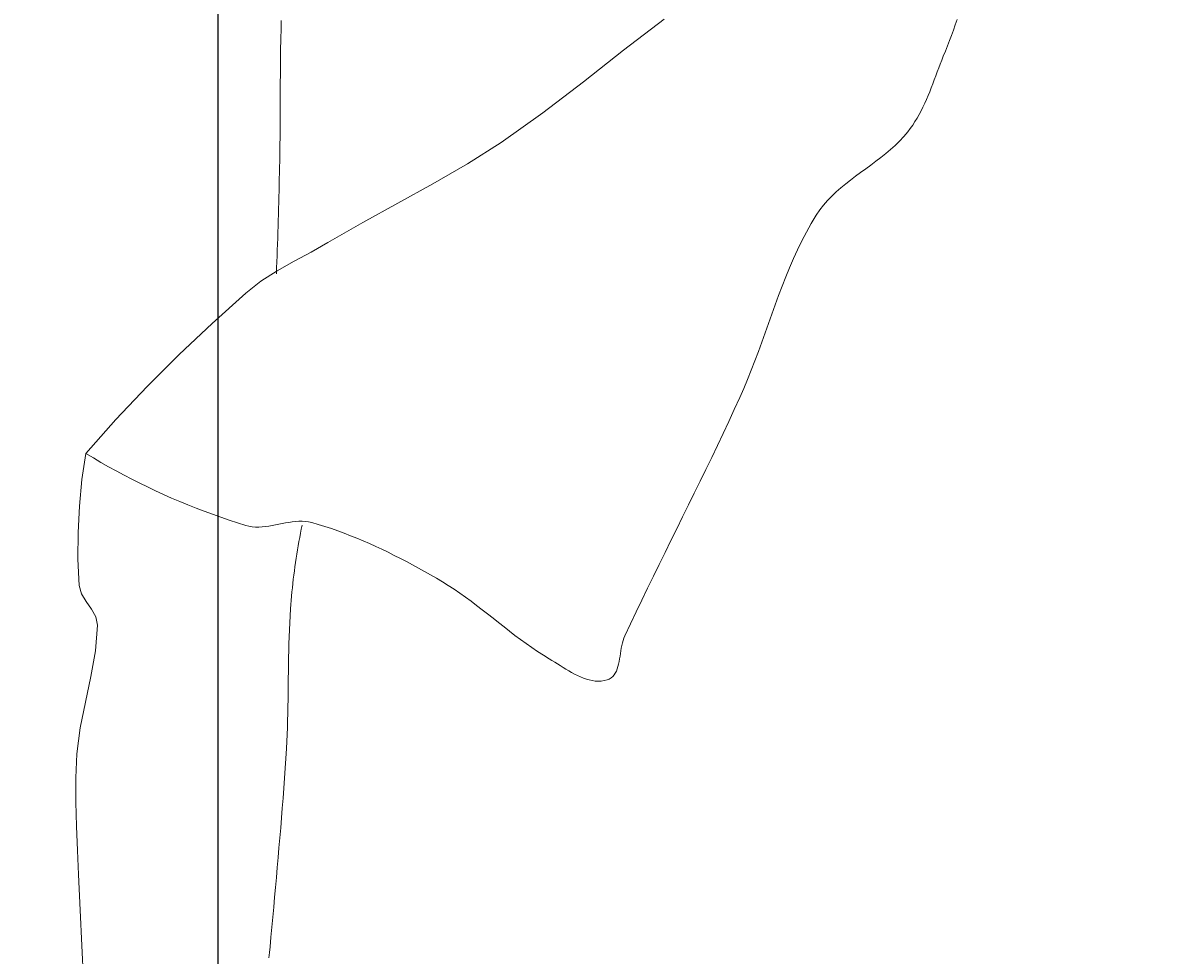
# Model space of a CAD drawing. Units: inches. Extents: x 1770 to 2988, y 1161 to 3221.
# Tile 25 of 44: x 2524 to 2562, y 2300 to 2330. Entities that reach past the tile are written whole.
import ezdxf

# ---------------------------------------------------------------- set-up
doc = ezdxf.new("R2010")
doc.units = ezdxf.units.IN
doc.layers.add('A-ANNO-DIMS', color=2, linetype='Continuous', lineweight=18)
doc.layers.add('A-FURN', color=8, linetype='Continuous', lineweight=13)
doc.styles.get("Standard").update_dxf_attribs({"font": 'arial.ttf'})
doc.dimstyles.get("Standard").update_dxf_attribs({"dimtxt": 0.18, "dimasz": 0.18, "dimexe": 0.18, "dimexo": 0.0625, "dimgap": 0.09, "dimtad": 0, "dimtih": 1, "dimtoh": 1, "dimdec": 4, "dimzin": 0, "dimdsep": 46, "dimtxsty": 'Standard', "dimcen": 0.09, "dimadec": 0, "dimazin": 0, "dimtfac": 1, "dimtdec": 4, "dimtofl": 0, "dimtmove": 0, "dimatfit": 3, "dimfxl": 1, "dimtolj": 1, "dimtzin": 0, "dimarcsym": 0})

# ---------------------------------------------------------------- blocks, each defined once
blk = doc.blocks.new('BED-DOUBLE-PLAN')
for p, q in [((6.794, 74.245), (6.798, 74.421)), ((6.798, 74.421), (6.803, 74.596)), ((19.481, 74.65), (18.14, 73.617)), ((29.058, 74.282), (29.122, 74.456)), ((29.122, 74.456), (29.185, 74.63)), ((6.786, 73.894), (6.79, 74.07)), ((6.79, 74.07), (6.794, 74.245)), ((28.927, 73.935), (28.993, 74.108)), ((28.993, 74.108), (29.058, 74.282)), ((6.779, 73.519), (6.782, 73.706)), ((6.782, 73.706), (6.786, 73.894)), ((28.792, 73.59), (28.86, 73.762)), ((28.86, 73.762), (28.927, 73.935)), ((6.775, 73.143), (6.777, 73.331)), ((6.777, 73.331), (6.779, 73.519)), ((18.14, 73.617), (16.81, 72.571)), ((28.623, 73.159), (28.673, 73.289)), ((28.673, 73.289), (28.724, 73.417)), ((28.724, 73.417), (28.792, 73.59)), ((6.772, 72.768), (6.773, 72.955)), ((6.773, 72.955), (6.775, 73.143)), ((28.476, 72.767), (28.525, 72.898)), ((28.525, 72.898), (28.574, 73.028)), ((28.574, 73.028), (28.623, 73.159)), ((6.77, 72.392), (6.771, 72.58)), ((6.771, 72.58), (6.772, 72.768)), ((16.81, 72.571), (15.466, 71.543)), ((28.327, 72.374), (28.377, 72.504)), ((28.377, 72.504), (28.427, 72.635)), ((28.427, 72.635), (28.476, 72.767)), ((6.769, 72.204), (6.77, 72.392)), ((6.769, 72.017), (6.769, 72.204)), ((28.168, 71.987), (28.222, 72.115)), ((28.222, 72.115), (28.275, 72.244)), ((28.275, 72.244), (28.327, 72.374)), ((6.767, 71.641), (6.768, 71.829)), ((6.768, 71.829), (6.769, 72.017)), ((27.99, 71.61), (28.052, 71.734)), ((28.052, 71.734), (28.111, 71.86)), ((28.111, 71.86), (28.168, 71.987)), ((6.766, 71.266), (6.767, 71.453)), ((6.767, 71.453), (6.767, 71.641)), ((15.466, 71.543), (14.086, 70.565)), ((27.786, 71.251), (27.858, 71.368)), ((27.858, 71.368), (27.926, 71.488)), ((27.926, 71.488), (27.99, 71.61)), ((6.763, 70.89), (6.765, 71.078)), ((6.765, 71.078), (6.766, 71.266)), ((27.547, 70.914), (27.631, 71.023)), ((27.631, 71.023), (27.711, 71.136)), ((27.711, 71.136), (27.786, 71.251)), ((6.759, 70.515), (6.762, 70.702)), ((6.762, 70.702), (6.763, 70.89)), ((27.128, 70.466), (27.275, 70.609)), ((27.275, 70.609), (27.415, 70.757)), ((27.415, 70.757), (27.547, 70.914)), ((6.754, 70.139), (6.757, 70.327)), ((6.757, 70.327), (6.759, 70.515)), ((14.086, 70.565), (12.968, 69.855)), ((26.817, 70.196), (26.975, 70.328)), ((26.975, 70.328), (27.128, 70.466)), ((6.746, 69.747), (6.75, 69.943)), ((6.75, 69.943), (6.754, 70.139)), ((12.968, 69.855), (11.823, 69.189)), ((26.324, 69.815), (26.491, 69.94)), ((26.491, 69.94), (26.655, 70.066)), ((26.655, 70.066), (26.817, 70.196)), ((6.737, 69.355), (6.742, 69.551)), ((6.742, 69.551), (6.746, 69.747)), ((25.82, 69.445), (25.988, 69.569)), ((25.988, 69.569), (26.156, 69.692)), ((26.156, 69.692), (26.324, 69.815)), ((6.728, 68.962), (6.733, 69.158)), ((6.733, 69.158), (6.737, 69.355)), ((11.823, 69.189), (10.663, 68.547)), ((25.335, 69.061), (25.493, 69.192)), ((25.493, 69.192), (25.655, 69.319)), ((25.655, 69.319), (25.82, 69.445)), ((6.718, 68.57), (6.723, 68.766)), ((6.723, 68.766), (6.728, 68.962)), ((24.892, 68.64), (25.033, 68.785)), ((25.033, 68.785), (25.181, 68.926)), ((25.181, 68.926), (25.335, 69.061)), ((6.708, 68.178), (6.713, 68.374)), ((6.713, 68.374), (6.718, 68.57)), ((10.663, 68.547), (9.501, 67.907)), ((24.52, 68.158), (24.635, 68.327)), ((24.635, 68.327), (24.759, 68.487)), ((24.759, 68.487), (24.892, 68.64)), ((6.696, 67.786), (6.702, 67.982)), ((6.702, 67.982), (6.708, 68.178)), ((24.35, 67.879), (24.52, 68.158)), ((6.684, 67.394), (6.69, 67.59)), ((6.69, 67.59), (6.696, 67.786)), ((9.501, 67.907), (8.35, 67.249)), ((24.039, 67.305), (24.19, 67.594)), ((24.19, 67.594), (24.35, 67.879)), ((6.671, 67.001), (6.678, 67.198)), ((6.678, 67.198), (6.684, 67.394)), ((8.35, 67.249), (7.792, 66.934)), ((23.895, 67.012), (24.039, 67.305)), ((6.657, 66.609), (6.664, 66.805)), ((6.664, 66.805), (6.671, 67.001)), ((7.792, 66.934), (7.227, 66.627)), ((23.759, 66.715), (23.895, 67.012)), ((6.65, 66.413), (6.657, 66.609)), ((7.227, 66.627), (6.669, 66.31)), ((23.629, 66.414), (23.759, 66.715)), ((6.669, 66.31), (6.131, 65.965)), ((6.643, 66.217), (6.65, 66.413)), ((23.385, 65.806), (23.505, 66.111)), ((23.505, 66.111), (23.629, 66.414)), ((6.131, 65.965), (5.627, 65.574)), ((23.268, 65.499), (23.385, 65.806)), ((5.627, 65.574), (4.51, 64.573)), ((23.155, 65.19), (23.268, 65.499)), ((23.043, 64.88), (23.155, 65.19)), ((4.51, 64.573), (3.42, 63.541)), ((22.823, 64.259), (22.933, 64.569)), ((22.933, 64.569), (23.043, 64.88)), ((22.712, 63.948), (22.823, 64.259)), ((22.6, 63.638), (22.712, 63.948)), ((3.42, 63.541), (2.36, 62.478)), ((22.485, 63.33), (22.6, 63.638)), ((22.245, 62.717), (22.367, 63.022)), ((22.367, 63.022), (22.485, 63.33)), ((22.119, 62.415), (22.245, 62.717)), ((2.36, 62.478), (1.33, 61.387)), ((21.986, 62.115), (22.119, 62.415)), ((21.803, 61.717), (21.986, 62.115)), ((21.619, 61.319), (21.803, 61.717)), ((1.33, 61.387), (0.332, 60.268)), ((21.432, 60.923), (21.619, 61.319)), ((21.244, 60.528), (21.432, 60.923)), ((21.055, 60.133), (21.244, 60.528)), ((0.332, 60.268), (0.204, 59.399)), ((0.332, 60.268), (0.58, 60.117)), ((0.58, 60.117), (0.831, 59.97)), ((0.831, 59.97), (1.084, 59.826)), ((20.864, 59.738), (21.055, 60.133)), ((1.084, 59.826), (1.339, 59.685)), ((1.339, 59.685), (1.596, 59.548)), ((20.672, 59.344), (20.864, 59.738)), ((0.204, 59.399), (0.118, 58.524)), ((1.596, 59.548), (1.854, 59.413)), ((1.854, 59.413), (2.114, 59.282)), ((2.114, 59.282), (2.376, 59.154)), ((20.48, 58.951), (20.672, 59.344)), ((2.376, 59.154), (2.64, 59.029)), ((2.64, 59.029), (2.905, 58.907)), ((2.905, 58.907), (3.172, 58.789)), ((20.287, 58.558), (20.48, 58.951)), ((0.118, 58.524), (0.073, 57.645)), ((3.172, 58.789), (3.44, 58.674)), ((3.44, 58.674), (3.709, 58.563)), ((3.709, 58.563), (3.98, 58.455)), ((3.98, 58.455), (4.252, 58.35)), ((20.093, 58.165), (20.287, 58.558)), ((4.252, 58.35), (4.525, 58.249)), ((4.525, 58.249), (4.8, 58.152)), ((4.8, 58.152), (5.075, 58.057)), ((19.899, 57.772), (20.093, 58.165)), ((5.075, 58.057), (5.352, 57.967)), ((5.352, 57.967), (5.629, 57.88)), ((5.629, 57.88), (5.734, 57.853)), ((5.734, 57.853), (5.84, 57.836)), ((5.84, 57.836), (5.948, 57.827)), ((5.948, 57.827), (6.056, 57.826)), ((6.056, 57.826), (6.165, 57.832)), ((6.165, 57.832), (6.275, 57.843)), ((6.275, 57.843), (6.386, 57.858)), ((6.386, 57.858), (6.496, 57.877)), ((6.496, 57.877), (6.608, 57.898)), ((6.608, 57.898), (6.719, 57.92)), ((6.719, 57.92), (6.83, 57.942)), ((6.83, 57.942), (6.941, 57.964)), ((6.941, 57.964), (7.052, 57.983)), ((7.052, 57.983), (7.163, 57.999)), ((7.163, 57.999), (7.273, 58.012)), ((7.273, 58.012), (7.383, 58.019)), ((7.383, 58.019), (7.492, 58.02)), ((7.467, 57.757), (7.44, 57.62)), ((7.495, 57.895), (7.467, 57.757)), ((7.492, 58.02), (7.6, 58.013)), ((7.6, 58.013), (7.707, 57.998)), ((7.707, 57.998), (7.813, 57.974)), ((7.813, 57.974), (8.03, 57.912)), ((8.03, 57.912), (8.246, 57.846)), ((8.246, 57.846), (8.461, 57.775)), ((8.461, 57.775), (8.675, 57.701)), ((8.675, 57.701), (8.887, 57.623)), ((19.705, 57.379), (19.899, 57.772)), ((0.073, 57.645), (0.07, 56.766)), ((7.388, 57.345), (7.363, 57.207)), ((7.413, 57.482), (7.388, 57.345)), ((7.44, 57.62), (7.413, 57.482)), ((8.887, 57.623), (9.098, 57.542)), ((9.098, 57.542), (9.308, 57.458)), ((9.308, 57.458), (9.517, 57.37)), ((9.517, 57.37), (9.725, 57.279)), ((19.512, 56.986), (19.705, 57.379)), ((7.317, 56.93), (7.296, 56.792)), ((7.34, 57.069), (7.317, 56.93)), ((7.363, 57.207), (7.34, 57.069)), ((9.725, 57.279), (9.932, 57.186)), ((9.932, 57.186), (10.138, 57.09)), ((10.138, 57.09), (10.342, 56.991)), ((10.342, 56.991), (10.546, 56.891)), ((19.318, 56.593), (19.512, 56.986)), ((0.07, 56.766), (0.108, 55.889)), ((7.275, 56.653), (7.255, 56.514)), ((7.296, 56.792), (7.275, 56.653)), ((10.546, 56.891), (10.748, 56.788)), ((10.748, 56.788), (10.95, 56.683)), ((10.95, 56.683), (11.15, 56.577)), ((11.15, 56.577), (11.349, 56.468)), ((19.125, 56.199), (19.318, 56.593)), ((7.218, 56.236), (7.201, 56.097)), ((7.236, 56.375), (7.218, 56.236)), ((7.255, 56.514), (7.236, 56.375)), ((11.349, 56.468), (11.548, 56.359)), ((11.548, 56.359), (11.745, 56.248)), ((11.745, 56.248), (11.942, 56.136)), ((18.933, 55.806), (19.125, 56.199)), ((0.108, 55.889), (0.185, 55.616)), ((7.17, 55.819), (7.156, 55.679)), ((7.185, 55.958), (7.17, 55.819)), ((7.201, 56.097), (7.185, 55.958)), ((11.942, 56.136), (12.139, 56.019)), ((12.139, 56.019), (12.334, 55.897)), ((12.334, 55.897), (12.525, 55.771)), ((18.742, 55.411), (18.933, 55.806)), ((0.185, 55.616), (0.338, 55.361)), ((7.143, 55.54), (7.131, 55.4)), ((7.156, 55.679), (7.143, 55.54)), ((12.525, 55.771), (12.714, 55.641)), ((12.714, 55.641), (12.901, 55.507)), ((12.901, 55.507), (13.086, 55.371)), ((18.552, 55.017), (18.742, 55.411)), ((0.338, 55.361), (0.515, 55.113)), ((0.515, 55.113), (0.66, 54.858)), ((7.109, 55.121), (7.094, 54.89)), ((7.119, 55.261), (7.109, 55.121)), ((7.131, 55.4), (7.119, 55.261)), ((13.086, 55.371), (13.27, 55.232)), ((13.27, 55.232), (13.452, 55.092)), ((13.452, 55.092), (13.634, 54.95)), ((0.66, 54.858), (0.717, 54.584)), ((7.081, 54.659), (7.071, 54.428)), ((7.094, 54.89), (7.081, 54.659)), ((13.634, 54.95), (13.815, 54.808)), ((13.815, 54.808), (13.996, 54.665)), ((13.996, 54.665), (14.178, 54.523)), ((18.364, 54.621), (18.552, 55.017)), ((0.717, 54.584), (0.65, 53.725)), ((7.071, 54.428), (7.062, 54.197)), ((14.178, 54.523), (14.36, 54.382)), ((14.36, 54.382), (14.542, 54.242)), ((18.176, 54.225), (18.364, 54.621)), ((7.055, 53.966), (7.05, 53.735)), ((7.062, 54.197), (7.055, 53.966)), ((14.542, 54.242), (14.727, 54.104)), ((14.727, 54.104), (14.912, 53.969)), ((14.912, 53.969), (15.1, 53.837)), ((18.062, 53.819), (18.078, 53.906)), ((18.078, 53.906), (18.097, 53.991)), ((18.097, 53.991), (18.12, 54.073)), ((18.12, 54.073), (18.146, 54.152)), ((18.146, 54.152), (18.176, 54.225)), ((0.65, 53.725), (0.501, 52.874)), ((7.05, 53.735), (7.045, 53.504)), ((15.1, 53.837), (15.29, 53.708)), ((15.29, 53.708), (15.483, 53.583)), ((15.483, 53.583), (15.679, 53.463)), ((18.005, 53.463), (18.019, 53.551)), ((18.019, 53.551), (18.033, 53.641)), ((18.033, 53.641), (18.047, 53.73)), ((18.047, 53.73), (18.062, 53.819)), ((7.041, 53.272), (7.038, 53.041)), ((7.045, 53.504), (7.041, 53.272)), ((15.679, 53.463), (15.767, 53.41)), ((15.767, 53.41), (15.856, 53.354)), ((15.856, 53.354), (15.947, 53.296)), ((15.947, 53.296), (16.039, 53.238)), ((16.039, 53.238), (16.132, 53.18)), ((16.132, 53.18), (16.227, 53.122)), ((17.926, 53.133), (17.951, 53.21)), ((17.951, 53.21), (17.971, 53.291)), ((17.971, 53.291), (17.989, 53.376)), ((17.989, 53.376), (18.005, 53.463)), ((0.501, 52.874), (0.318, 52.025)), ((7.036, 52.81), (7.033, 52.578)), ((7.038, 53.041), (7.036, 52.81)), ((16.227, 53.122), (16.322, 53.065)), ((16.322, 53.065), (16.417, 53.011)), ((16.417, 53.011), (16.514, 52.959)), ((16.514, 52.959), (16.611, 52.91)), ((16.611, 52.91), (16.709, 52.866)), ((16.709, 52.866), (16.807, 52.826)), ((16.807, 52.826), (16.905, 52.792)), ((16.905, 52.792), (17.003, 52.764)), ((17.003, 52.764), (17.102, 52.743)), ((17.495, 52.743), (17.593, 52.767)), ((17.593, 52.767), (17.664, 52.795)), ((17.664, 52.795), (17.725, 52.832)), ((17.725, 52.832), (17.779, 52.878)), ((17.779, 52.878), (17.825, 52.932)), ((17.825, 52.932), (17.864, 52.993)), ((17.864, 52.993), (17.898, 53.06)), ((17.898, 53.06), (17.926, 53.133)), ((7.033, 52.578), (7.03, 52.347)), ((17.102, 52.743), (17.201, 52.73)), ((17.201, 52.73), (17.299, 52.725)), ((17.299, 52.725), (17.397, 52.729)), ((17.397, 52.729), (17.495, 52.743)), ((0.318, 52.025), (0.148, 51.175)), ((7.027, 52.116), (7.024, 51.884)), ((7.03, 52.347), (7.027, 52.116)), ((7.019, 51.653), (7.013, 51.422)), ((7.024, 51.884), (7.019, 51.653)), ((7.013, 51.422), (7.006, 51.19)), ((0.148, 51.175), (0.038, 50.318)), ((6.997, 50.959), (6.987, 50.728)), ((7.006, 51.19), (6.997, 50.959)), ((6.974, 50.497), (6.954, 50.168)), ((6.987, 50.728), (6.974, 50.497)), ((0.038, 50.318), (0, 49.52)), ((6.954, 50.168), (6.932, 49.839)), ((6.932, 49.839), (6.909, 49.51)), ((0, 49.52), (0, 48.719)), ((6.909, 49.51), (6.886, 49.182)), ((6.886, 49.182), (6.861, 48.853)), ((0, 48.719), (0.024, 47.919)), ((6.861, 48.853), (6.836, 48.524)), ((6.836, 48.524), (6.809, 48.195)), ((0.024, 47.919), (0.059, 47.118)), ((6.783, 47.867), (6.755, 47.538)), ((6.809, 48.195), (6.783, 47.867)), ((6.755, 47.538), (6.727, 47.209)), ((0.059, 47.118), (0.094, 46.318)), ((6.727, 47.209), (6.698, 46.881)), ((6.698, 46.881), (6.669, 46.552)), ((0.094, 46.318), (0.141, 45.147)), ((6.669, 46.552), (6.64, 46.224)), ((6.64, 46.224), (6.611, 45.896)), ((6.581, 45.567), (6.551, 45.239)), ((6.611, 45.896), (6.581, 45.567)), ((6.551, 45.239), (6.522, 44.91)), ((0.141, 45.147), (0.197, 43.977)), ((6.522, 44.91), (6.492, 44.582)), ((6.492, 44.582), (6.462, 44.253)), ((6.462, 44.253), (6.433, 43.925)), ((0.197, 43.977), (0.26, 42.807)), ((6.415, 43.745), (6.396, 43.565)), ((6.433, 43.925), (6.415, 43.745))]:
    blk.add_line(p, q)
blk = doc.blocks.new('*D82')
at = {"layer": 'A-ANNO-DIMS', "color": 0, "lineweight": -2, "transparency": 16777216}
for p, q in [((2443.386, 1610.265), (2443.386, 2570.705)), ((2443.566, 2570.525), (2486.452, 2570.525)), ((2530.124, 2570.525), (2487.238, 2570.525)), ((2530.304, 1610.265), (2530.304, 2570.705))]:
    blk.add_line(p, q, dxfattribs=at)
at = {"layer": 'A-ANNO-DIMS', "color": 0, "transparency": 16777216}
for points in [[(2443.566, 2570.555), (2443.566, 2570.495), (2443.386, 2570.525)], [(2530.124, 2570.555), (2530.124, 2570.495), (2530.304, 2570.525)]]:
    blk.add_solid(points, dxfattribs=at)
at = {"layer": 'Defpoints', "color": 0, "transparency": 16777216}
for p in [(2530.304, 2570.525), (2443.386, 1610.202), (2530.304, 1610.202)]:
    blk.add_point(p, dxfattribs=at)
at = {"layer": 'A-ANNO-DIMS', "color": 0, "transparency": 16777216, "insert": (2486.845, 2570.525), "char_height": 0.18, "attachment_point": 5}
blk.add_mtext('\\A1;86.92', dxfattribs=at)
blk = doc.blocks.new('*D84')
at = {"layer": 'A-ANNO-DIMS', "color": 0, "lineweight": -2, "transparency": 16777216}
for p, q in [((2513.196, 1835.265), (2513.196, 2570.705)), ((2513.376, 2570.525), (2564.56, 2570.525)), ((2616.516, 2570.525), (2565.332, 2570.525)), ((2616.696, 1835.265), (2616.696, 2570.705))]:
    blk.add_line(p, q, dxfattribs=at)
at = {"layer": 'A-ANNO-DIMS', "color": 0, "transparency": 16777216}
for points in [[(2513.376, 2570.555), (2513.376, 2570.495), (2513.196, 2570.525)], [(2616.516, 2570.555), (2616.516, 2570.495), (2616.696, 2570.525)]]:
    blk.add_solid(points, dxfattribs=at)
at = {"layer": 'Defpoints', "color": 0, "transparency": 16777216}
for p in [(2616.696, 2570.525), (2513.196, 1835.202), (2616.696, 1835.202)]:
    blk.add_point(p, dxfattribs=at)
at = {"layer": 'A-ANNO-DIMS', "color": 0, "transparency": 16777216, "insert": (2564.946, 2570.525), "char_height": 0.18, "attachment_point": 5}
blk.add_mtext('\\A1;103.5', dxfattribs=at)

msp = doc.modelspace()

# ---------------------------------------------------------------- block references
at = {"layer": 'A-FURN'}
msp.add_blockref('BED-DOUBLE-PLAN', (2525.5949, 2255.9126), dxfattribs=at)

# ---------------------------------------------------------------- dimensions: what is measured, and where the dimension line sits
at = {"layer": 'A-ANNO-DIMS'}
for base, p1, p2, override, picture, middle in [((2530.3038, 2570.5247), (2443.3863, 1610.2021), (2530.3038, 1610.2021), {"dimdec": 2, "dimlfac": 1, "dimrnd": 0, "dimzin": 0, "dimdsep": 46, "dimlunit": 2}, '*D82', (2486.8451, 2570.5247)), ((2616.696, 2570.5247), (2513.196, 1835.2021), (2616.696, 1835.2021), {"dimdec": 1, "dimlfac": 1, "dimrnd": 0, "dimzin": 0, "dimdsep": 46, "dimlunit": 2}, '*D84', (2564.946, 2570.5247))]:
    dim = msp.add_linear_dim(base=base, p1=p1, p2=p2, dimstyle='Standard', override=override, dxfattribs=at)
    dim.commit()
    dim.dimension.update_dxf_attribs({"geometry": picture, "text_midpoint": middle})

doc.saveas('drawing.dxf')
